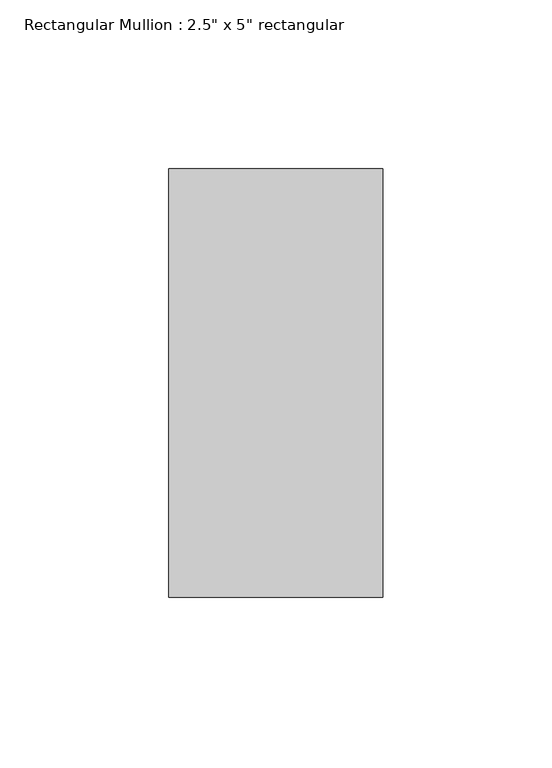
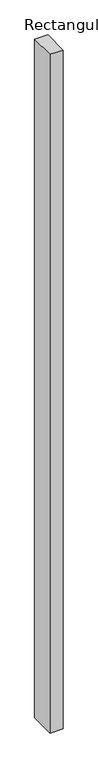
"""IFC4 building model written with IfcOpenShell, lengths in millimetres: member geometry."""

from ifc_helpers import new_model, si_unit, frame, origin, place, context, project, spatial, polyline, outline, extrude, source, transform, mapped, element, save


def member_9c8919e3(model_context):
    return source(origin(), model_context, "Body", "SweptSolid", [
        extrude(outline(polyline([(0.0, 63.5), (0.0, -63.5), (-63.5, -63.5), (-63.5, 63.5), (0.0, 63.5)])), frame((0.0, 0.0, -3454.61006), z_axis=(0.0, 0.0, 1.0), x_axis=(1.0, 0.0, 0.0)), (0.0, 0.0, 1.0), 3454.61006),
    ])


if __name__ == "__main__":
    model = new_model("IFC4")
    model_context = context("Model", 3, world=origin())
    ifc_project = project(units=[si_unit("LENGTHUNIT", "METRE", prefix="MILLI")], contexts=[model_context])
    site = spatial("IfcSite", under=ifc_project)
    building = spatial("IfcBuilding", under=site)
    placement = place(None, origin())
    member_shape = member_9c8919e3(model_context)
    element("IfcMember", 1, ObjectType="Rectangular Mullion : 2.5\" x 5\" rectangular", at=placement, inside=building, context=model_context, shape_type="MappedRepresentation", body=[
        mapped(member_shape, transform((0.0, 0.0, 0.0), x_axis=(1.0, 0.0, 0.0), y_axis=(0.0, 1.0, 0.0), z_axis=(0.0, 0.0, 1.0))),
    ])
    save(model, "model.ifc")

# Revit data of these elements
# Type "Rectangular Mullion : 2.5\" x 5\" rectangular"
#   built-in parameter 1007304 = 0.416667 (stored number, unit not read)
#   built-in parameter 1007301 = 0.104167 (stored number, unit not read)
#   built-in parameter 1007300 = 0.104167 (stored number, unit not read)
# Element 1 (IfcMember, "Rectangular Mullion : 2.5\" x 5\" rectangular")
#   Materials on its faces: "Aluminum"
# Materials
#   "Aluminum": class "Metal", colour RGB 247 247 247, transparency 0, Description = "Aluminum 6061", Cost = 0
